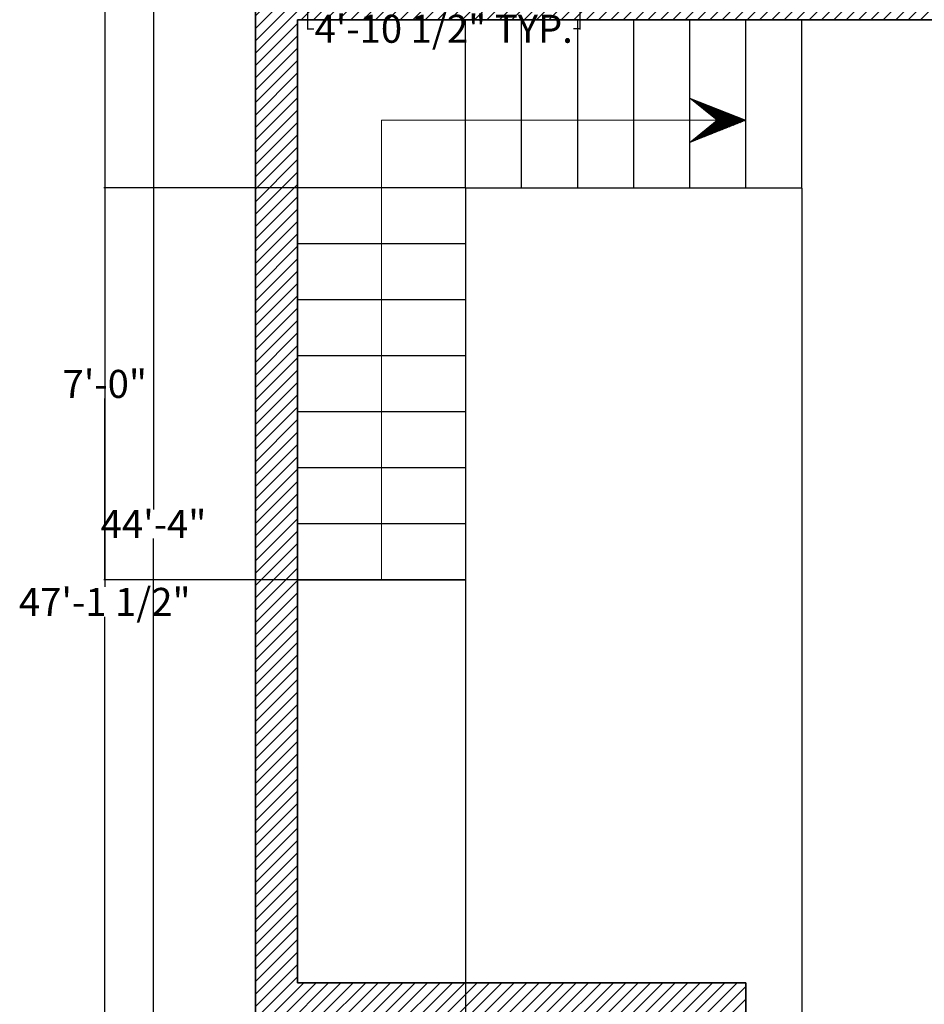
# Model space of a CAD drawing. Units: inches. Extents: x 585 to 1401, y -184 to 463.
# Tile 3 of 8: x 604 to 798, y 53 to 264. Entities that reach past the tile are written whole.
import ezdxf

# ---------------------------------------------------------------- set-up
doc = ezdxf.new("R2010")
doc.units = ezdxf.units.IN
doc.header["$MEASUREMENT"] = 0
for name, color, linetype, lineweight in [('A-ANNO-DIMS', 2, 'Continuous', 18), ('A-ANNO-SYMB', 4, 'Continuous', 18), ('A-Wall', 7, 'Continuous', 35), ('A-WALL-PATT', 252, 'Continuous', 13), ('STAIRS', 4, 'Continuous', 25)]:
    doc.layers.add(name, color=color, linetype=linetype, lineweight=lineweight)
doc.styles.get("Standard").update_dxf_attribs({"font": 'arial.ttf'})
doc.dimstyles.get("Standard").update_dxf_attribs({"dimtxt": 6, "dimasz": 0.18, "dimexe": 0.18, "dimexo": 0.0625, "dimgap": 0.09, "dimtad": 0, "dimtih": 1, "dimtoh": 1, "dimdec": 0, "dimzin": 0, "dimdsep": 46, "dimlunit": 3, "dimtxsty": 'Standard', "dimblk": 'ARCHTICK', "dimcen": 0.09, "dimadec": 0, "dimazin": 0, "dimtfac": 1, "dimtdec": 0, "dimtofl": 0, "dimtmove": 0, "dimatfit": 3, "dimfxl": 1, "dimtolj": 1, "dimtzin": 0, "dimarcsym": 0})

# ---------------------------------------------------------------- blocks, each defined once
blk = doc.blocks.new('_ArchTick')
at = {"color": 0, "linetype": 'ByBlock', "const_width": 0.15}
blk.add_lwpolyline([(-0.5, -0.5), (0.5, 0.5)], dxfattribs=at)
blk = doc.blocks.new('*D27')
at = {"layer": 'A-ANNO-DIMS', "color": 0, "lineweight": -2, "transparency": 16777216}
for p, q in [((654.47, 422.15), (632.54, 422.15)), ((632.72, 422.15), (632.72, 159.24)), ((632.72, -109.85), (632.72, 153.06)), ((654.47, -109.85), (632.54, -109.85))]:
    blk.add_line(p, q, dxfattribs=at)
at = {"layer": 'Defpoints', "color": 0, "transparency": 16777216}
for p in [(654.53, 422.15), (632.72, -109.85), (654.53, -109.85)]:
    blk.add_point(p, dxfattribs=at)
at = {"layer": 'A-ANNO-DIMS', "color": 0, "lineweight": -2, "transparency": 16777216, "xscale": 0.18, "yscale": 0.18, "zscale": 0.18}
for p, rotation in [((632.72, 422.15), 90), ((632.72, -109.85), 270)]:
    blk.add_blockref('_ArchTick', p, dxfattribs=dict(at, rotation=rotation))
at = {"layer": 'A-ANNO-DIMS', "color": 0, "transparency": 16777216, "insert": (632.72, 156.15), "char_height": 6, "attachment_point": 5}
blk.add_mtext('\\A1;44\'-4"', dxfattribs=at)
blk = doc.blocks.new('*D65')
at = {"layer": 'A-ANNO-DIMS', "color": 0, "lineweight": -2, "transparency": 16777216}
for p, q in [((665.71, 271.32), (665.71, 262.03)), ((723.97, 271.32), (723.97, 262.03)), ((665.71, 262.21), (667.02, 262.21)), ((723.97, 262.21), (722.66, 262.21))]:
    blk.add_line(p, q, dxfattribs=at)
at = {"layer": 'Defpoints', "color": 0, "transparency": 16777216}
for p in [(665.71, 271.38), (723.97, 271.38), (723.97, 262.21)]:
    blk.add_point(p, dxfattribs=at)
at = {"layer": 'A-ANNO-DIMS', "color": 0, "lineweight": -2, "transparency": 16777216, "xscale": 0.18, "yscale": 0.18, "zscale": 0.18, "rotation": 180}
blk.add_blockref('_ArchTick', (665.71, 262.21), dxfattribs=at)
at = {"layer": 'A-ANNO-DIMS', "color": 0, "lineweight": -2, "transparency": 16777216, "xscale": 0.18, "yscale": 0.18, "zscale": 0.18}
blk.add_blockref('_ArchTick', (723.97, 262.21), dxfattribs=at)
at = {"layer": 'A-ANNO-DIMS', "color": 0, "transparency": 16777216, "insert": (694.84, 262.21), "char_height": 6, "attachment_point": 5}
blk.add_mtext('\\A1;4\'-10 1/2" TYP.', dxfattribs=at)
blk = doc.blocks.new('*D70')
at = {"layer": 'A-ANNO-DIMS', "color": 0, "lineweight": -2, "transparency": 16777216}
for p, q in [((665.71, 27.87), (665.71, 42.68)), ((665.71, 42.5), (671.34, 42.5)), ((763.62, 42.5), (757.99, 42.5)), ((763.62, 27.87), (763.62, 42.68))]:
    blk.add_line(p, q, dxfattribs=at)
at = {"layer": 'Defpoints', "color": 0, "transparency": 16777216}
for p in [(763.62, 42.5), (665.71, 27.81), (763.62, 27.81)]:
    blk.add_point(p, dxfattribs=at)
at = {"layer": 'A-ANNO-DIMS', "color": 0, "lineweight": -2, "transparency": 16777216, "xscale": 0.18, "yscale": 0.18, "zscale": 0.18, "rotation": 180}
blk.add_blockref('_ArchTick', (665.71, 42.5), dxfattribs=at)
at = {"layer": 'A-ANNO-DIMS', "color": 0, "lineweight": -2, "transparency": 16777216, "xscale": 0.18, "yscale": 0.18, "zscale": 0.18}
blk.add_blockref('_ArchTick', (763.62, 42.5), dxfattribs=at)
at = {"layer": 'A-ANNO-DIMS', "color": 0, "transparency": 16777216, "insert": (714.67, 42.5), "char_height": 6, "attachment_point": 5}
blk.add_mtext('\\A1;LOUNGE GROUP 8\'-2"', dxfattribs=at)
blk = doc.blocks.new('*D76')
at = {"layer": 'A-ANNO-DIMS', "color": 0, "lineweight": -2, "transparency": 16777216}
for p, q in [((654.47, 422.15), (622.1, 422.15)), ((622.28, 422.15), (622.28, 142.65)), ((622.28, -143.23), (622.28, 136.27)), ((807.47, -143.23), (622.1, -143.23))]:
    blk.add_line(p, q, dxfattribs=at)
at = {"layer": 'Defpoints', "color": 0, "transparency": 16777216}
for p in [(622.28, 422.15), (654.53, 422.15), (807.53, -143.23)]:
    blk.add_point(p, dxfattribs=at)
at = {"layer": 'A-ANNO-DIMS', "color": 0, "lineweight": -2, "transparency": 16777216, "xscale": 0.18, "yscale": 0.18, "zscale": 0.18}
for p, rotation in [((622.28, 422.15), 90), ((622.28, -143.23), 270)]:
    blk.add_blockref('_ArchTick', p, dxfattribs=dict(at, rotation=rotation))
at = {"layer": 'A-ANNO-DIMS', "color": 0, "transparency": 16777216, "insert": (622.28, 139.46), "char_height": 6, "attachment_point": 5}
blk.add_mtext('\\A1;47\'-1 1/2"', dxfattribs=at)
blk = doc.blocks.new('*D80')
at = {"layer": 'A-ANNO-DIMS', "color": 0, "lineweight": -2, "transparency": 16777216}
for p, q in [((699.47, 228.15), (622.1, 228.15)), ((622.28, 228.15), (622.28, 189.31)), ((622.28, 144.15), (622.28, 183)), ((699.47, 144.15), (622.1, 144.15))]:
    blk.add_line(p, q, dxfattribs=at)
at = {"layer": 'Defpoints', "color": 0, "transparency": 16777216}
for p in [(622.28, 228.15), (699.53, 228.15), (699.53, 144.15)]:
    blk.add_point(p, dxfattribs=at)
at = {"layer": 'A-ANNO-DIMS', "color": 0, "lineweight": -2, "transparency": 16777216, "xscale": 0.18, "yscale": 0.18, "zscale": 0.18}
for p, rotation in [((622.28, 228.15), 90), ((622.28, 144.15), 270)]:
    blk.add_blockref('_ArchTick', p, dxfattribs=dict(at, rotation=rotation))
at = {"layer": 'A-ANNO-DIMS', "color": 0, "transparency": 16777216, "insert": (622.28, 186.15), "char_height": 6, "attachment_point": 5}
blk.add_mtext('\\A1;7\'-0"', dxfattribs=at)
blk = doc.blocks.new('*D81')
at = {"layer": 'A-ANNO-DIMS', "color": 0, "lineweight": -2, "transparency": 16777216}
for p, q in [((699.53, 228.09), (699.53, -175.66)), ((771.53, 228.09), (771.53, -175.66)), ((699.53, -175.48), (727.45, -175.48)), ((771.53, -175.48), (743.61, -175.48))]:
    blk.add_line(p, q, dxfattribs=at)
at = {"layer": 'Defpoints', "color": 0, "transparency": 16777216}
for p in [(699.53, 228.15), (771.53, 228.15), (771.53, -175.48)]:
    blk.add_point(p, dxfattribs=at)
at = {"layer": 'A-ANNO-DIMS', "color": 0, "lineweight": -2, "transparency": 16777216, "xscale": 0.18, "yscale": 0.18, "zscale": 0.18, "rotation": 180}
blk.add_blockref('_ArchTick', (699.53, -175.48), dxfattribs=at)
at = {"layer": 'A-ANNO-DIMS', "color": 0, "lineweight": -2, "transparency": 16777216, "xscale": 0.18, "yscale": 0.18, "zscale": 0.18}
blk.add_blockref('_ArchTick', (771.53, -175.48), dxfattribs=at)
at = {"layer": 'A-ANNO-DIMS', "color": 0, "transparency": 16777216, "insert": (735.53, -175.48), "char_height": 6, "attachment_point": 5}
blk.add_mtext('\\A1;6\'-0"', dxfattribs=at)

msp = doc.modelspace()

# ---------------------------------------------------------------- hatches: boundary and pattern name
at = {"layer": 'A-ANNO-SYMB'}
h = msp.add_hatch(dxfattribs=at)
h.set_pattern_fill('ANSI31', color=256)
h.set_pattern_definition([(45, (599.059, -1e-14), (-0.08838835, 0.08838835), [])])
h.paths.add_polyline_path([(759.53, 242.6), (747.53, 247.34), (753.4, 242.6), (747.53, 237.86)])
at = {"layer": 'A-WALL-PATT'}
h = msp.add_hatch(dxfattribs=at)
h.set_pattern_fill('ANSI31', color=256, scale=15)
h.set_pattern_definition([(45, (599.059, -1e-14), (-1.325825, 1.325825), [])])
h.paths.add_polyline_path([(711.53, 422.15), (654.53, 422.15), (654.53, -109.85), (680.03, -109.85), (680.03, -100.85), (663.53, -100.85), (663.53, 48.87), (759.53, 48.87), (759.53, 57.87), (663.53, 57.87), (663.53, 144.15), (663.53, 264.15), (812.53, 264.15), (812.53, 269.15), (663.53, 269.15), (663.53, 413.15), (711.53, 413.15)])
h.paths.add_polyline_path([(753.53, -100.85), (728.03, -100.85), (728.03, -109.85), (753.53, -109.85)], flags=17)
h.paths.add_polyline_path([(812.53, -71.54), (807.53, -71.54), (807.53, -100.85), (795.53, -100.85), (795.53, -109.85), (807.53, -109.85), (807.53, -143.23), (848.53, -143.23), (848.53, -134.23), (812.53, -134.23)])
h.paths.add_polyline_path([(941.53, 8.77), (932.53, 8.77), (932.53, -9.23), (812.53, -9.23), (812.53, 5.77), (807.53, 5.77), (807.53, -29.54), (812.53, -29.54), (812.53, -14.23), (932.53, -14.23), (932.53, -134.23), (896.53, -134.23), (896.53, -143.23), (941.53, -143.23)])
h.paths.add_polyline_path([(941.53, 91.77), (932.53, 91.77), (932.53, 55.77), (812.53, 55.77), (812.53, 98.58), (807.53, 98.58), (807.53, 35.77), (812.53, 35.77), (812.53, 50.77), (932.53, 50.77), (932.53, 32.77), (941.53, 32.77)])
h.paths.add_polyline_path([(941.53, 222.04), (932.53, 222.04), (932.53, 180.77), (807.53, 180.77), (807.53, 140.58), (812.53, 140.58), (812.53, 175.77), (932.53, 175.77), (932.53, 139.77), (941.53, 139.77)])
h.paths.add_polyline_path([(941.53, 422.15), (896.53, 422.15), (896.53, 413.15), (932.53, 413.15), (932.53, 317.15), (896.53, 317.15), (896.53, 312.15), (932.53, 312.15), (932.53, 270.04), (941.53, 270.04)])
h.paths.add_polyline_path([(848.53, 422.15), (759.53, 422.15), (759.53, 413.15), (807.53, 413.15), (807.53, 312.15), (848.53, 312.15), (848.53, 317.15), (812.53, 317.15), (812.53, 413.15), (848.53, 413.15)])

# ---------------------------------------------------------------- linework, layer by layer
at = {"layer": 'A-ANNO-SYMB'}
for p, q in [((753.4, 242.6), (747.53, 247.34)), ((747.53, 247.34), (759.53, 242.6)), ((681.53, 144.15), (681.53, 242.6)), ((681.53, 242.6), (753.4, 242.6)), ((753.4, 242.6), (747.53, 237.86)), ((747.53, 237.86), (759.53, 242.6))]:
    msp.add_line(p, q, dxfattribs=at)
at = {"layer": 'A-Wall'}
for p, q in [((654.53, 422.15), (654.53, -109.85)), ((663.53, 264.15), (812.53, 264.15)), ((663.53, 264.15), (663.53, 144.15)), ((663.53, 144.15), (663.53, 57.87)), ((759.53, 57.87), (663.53, 57.87)), ((759.53, 57.87), (759.53, 48.87))]:
    msp.add_line(p, q, dxfattribs=at)
at = {"layer": 'STAIRS'}
for p, q in [((699.53, 228.15), (699.53, 264.15)), ((711.53, 228.15), (711.53, 264.15)), ((723.53, 228.15), (723.53, 264.15)), ((735.53, 228.15), (735.53, 264.15)), ((747.53, 228.15), (747.53, 264.15)), ((759.53, 228.15), (759.53, 264.15)), ((771.53, 228.15), (771.53, 264.15)), ((699.53, 228.15), (663.53, 228.15)), ((699.53, 228.15), (699.53, 144.15)), ((699.53, 228.15), (771.53, 228.15)), ((699.53, 216.15), (663.53, 216.15)), ((699.53, 204.15), (663.53, 204.15)), ((699.53, 192.15), (663.53, 192.15)), ((699.53, 180.15), (663.53, 180.15)), ((699.53, 168.15), (663.53, 168.15)), ((699.53, 156.15), (663.53, 156.15)), ((663.53, 144.15), (699.53, 144.15)), ((699.53, 144.15), (663.53, 144.15))]:
    msp.add_line(p, q, dxfattribs=at)

# ---------------------------------------------------------------- dimensions: what is measured, and where the dimension line sits
at = {"layer": 'A-ANNO-DIMS'}
for base, p1, p2, override, picture, middle in [((622.28, 422.15), (807.53, -143.23), (654.53, 422.15), {"dimdec": 1, "dimlfac": 1, "dimrnd": 0, "dimzin": 1, "dimdsep": 46, "dimlunit": 4, "dimfrac": 2}, '*D76', (622.28, 139.46)), ((632.72, -109.85), (654.53, 422.15), (654.53, -109.85), {"dimclrd": 0, "dimclre": 0, "dimclrt": 0}, '*D27', (632.72, 156.15)), ((622.28, 228.15), (699.53, 144.15), (699.53, 228.15), {"dimdec": 1, "dimlfac": 1, "dimrnd": 0, "dimzin": 1, "dimdsep": 46, "dimlunit": 4, "dimfrac": 2}, '*D80', (622.28, 186.15))]:
    dim = msp.add_linear_dim(base=base, p1=p1, p2=p2, angle=90, dimstyle='Standard', override=override, dxfattribs=at)
    dim.commit()
    dim.dimension.update_dxf_attribs({"geometry": picture, "text_midpoint": middle})
for base, p1, p2, text, picture, middle in [((723.97, 262.21), (665.71, 271.38), (723.97, 271.38), '<> TYP.', '*D65', (694.84, 262.21)), ((763.62, 42.5), (665.71, 27.81), (763.62, 27.81), 'LOUNGE GROUP <>', '*D70', (714.67, 42.5))]:
    dim = msp.add_linear_dim(base=base, p1=p1, p2=p2, text=text, dimstyle='Standard', override={"dimdec": 1, "dimlfac": 1, "dimrnd": 0, "dimzin": 1, "dimdsep": 46, "dimlunit": 4, "dimfrac": 2}, dxfattribs=at)
    dim.commit()
    dim.dimension.update_dxf_attribs({"geometry": picture, "text_midpoint": middle})
dim = msp.add_linear_dim(base=(771.53, -175.48), p1=(699.53, 228.15), p2=(771.53, 228.15), dimstyle='Standard', override={"dimdec": 1, "dimlfac": 1, "dimrnd": 0, "dimzin": 1, "dimdsep": 46, "dimlunit": 4, "dimfrac": 2}, dxfattribs=at)
dim.commit()
dim.dimension.update_dxf_attribs({"geometry": '*D81', "text_midpoint": (735.53, -175.48)})

doc.saveas('drawing.dxf')
